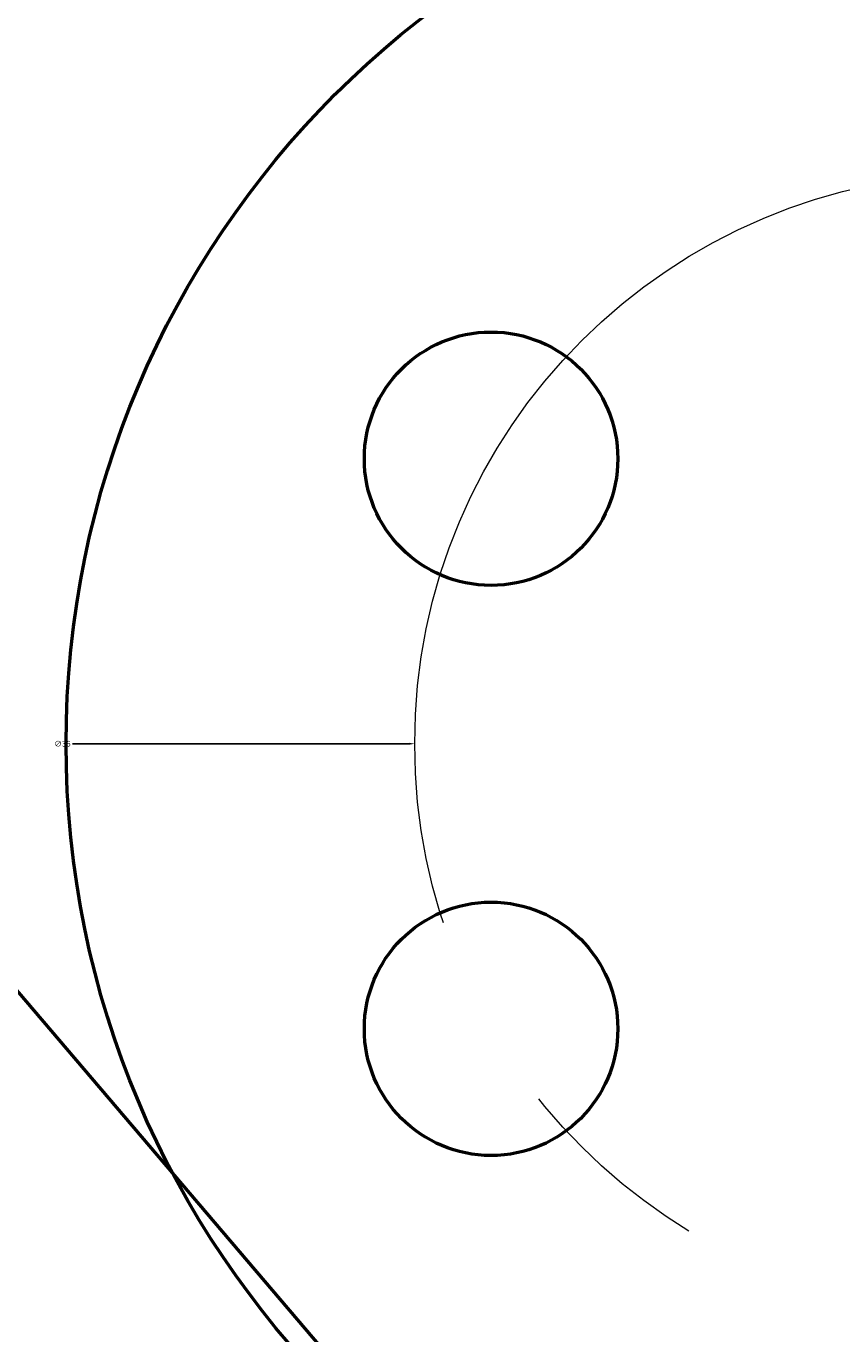
# Model space of a CAD drawing. Units: inches. Extents: x -11 to 126, y -62 to 82.
# Tile 3 of 10: x 29 to 55, y -40 to 1. Entities that reach past the tile are written whole.
import ezdxf

# ---------------------------------------------------------------- set-up
doc = ezdxf.new("R2010")
doc.units = ezdxf.units.IN
doc.header["$MEASUREMENT"] = 0
doc.linetypes.add('CENTER', pattern=[50.8, 31.75, -6.35, 6.35, -6.35])
for name, color, linetype, lineweight in [('M-CNTR', 4, 'CENTER', 18), ('M-DIMS', 2, 'Continuous', 18), ('M-OUTL', 7, 'Continuous', 50)]:
    doc.layers.add(name, color=color, linetype=linetype, lineweight=lineweight)
doc.styles.get("Standard").update_dxf_attribs({"font": 'arial.ttf'})
doc.dimstyles.get("Standard").update_dxf_attribs({"dimtxt": 0.18, "dimasz": 0.18, "dimexe": 0.18, "dimexo": 0.0625, "dimgap": 0.09, "dimtad": 0, "dimtih": 1, "dimtoh": 1, "dimdec": 4, "dimzin": 0, "dimdsep": 46, "dimtxsty": 'Standard', "dimcen": 0.09, "dimadec": 0, "dimazin": 0, "dimtfac": 1, "dimtdec": 4, "dimtofl": 0, "dimtmove": 0, "dimatfit": 3, "dimfxl": 1, "dimtolj": 1, "dimtzin": 0, "dimarcsym": 0})

# ---------------------------------------------------------------- blocks, each defined once
blk = doc.blocks.new('*U3')
blk.add_circle((0, 0), 4)
blk = doc.blocks.new('*U4')
at = {"layer": 'M-OUTL', "color": 0, "linetype": 'ByBlock', "lineweight": -2, "transparency": 16777216}
for p, rotation in [((43.643, -12.646), 59.99999999999999), ((43.643, -30.646), 120)]:
    blk.add_blockref('*U3', p, dxfattribs=dict(at, rotation=rotation))
blk = doc.blocks.new('*D5')
at = {"layer": 'Defpoints', "color": 0, "transparency": 16777216}
for p in [(119.232, 12.354), (-0.749, 11.479), (119.232, -57.296)]:
    blk.add_point(p, dxfattribs=at)
at = {"layer": 'M-DIMS', "color": 0, "lineweight": -2, "transparency": 16777216}
for p, q in [((119.232, 12.292), (119.232, -57.476)), ((-0.749, 11.416), (-0.749, -57.476)), ((-0.569, -57.296), (58.786, -57.296)), ((119.052, -57.296), (59.696, -57.296))]:
    blk.add_line(p, q, dxfattribs=at)
at = {"layer": 'M-DIMS', "color": 0, "transparency": 16777216}
for points in [[(-0.569, -57.266), (-0.569, -57.326), (-0.749, -57.296)], [(119.052, -57.266), (119.052, -57.326), (119.232, -57.296)]]:
    blk.add_solid(points, dxfattribs=at)
at = {"layer": 'M-DIMS', "color": 0, "transparency": 16777216, "insert": (59.241, -57.296), "char_height": 0.18, "attachment_point": 5}
blk.add_mtext('\\A1;119.98', dxfattribs=at)
blk = doc.blocks.new('*D6')
at = {"layer": 'Defpoints', "color": 0, "transparency": 16777216}
for p in [(-7.399, 75.354), (59.232, 75.354), (59.232, -50.646)]:
    blk.add_point(p, dxfattribs=at)
at = {"layer": 'M-DIMS', "color": 0, "lineweight": -2, "transparency": 16777216}
for p, q in [((59.169, 75.354), (-7.579, 75.354)), ((-7.399, 75.174), (-7.399, 12.536)), ((-7.399, -50.466), (-7.399, 12.172)), ((59.169, -50.646), (-7.579, -50.646))]:
    blk.add_line(p, q, dxfattribs=at)
at = {"layer": 'M-DIMS', "color": 0, "transparency": 16777216}
for points in [[(-7.429, 75.174), (-7.369, 75.174), (-7.399, 75.354)], [(-7.429, -50.466), (-7.369, -50.466), (-7.399, -50.646)]]:
    blk.add_solid(points, dxfattribs=at)
at = {"layer": 'M-DIMS', "color": 0, "transparency": 16777216, "insert": (-7.399, 12.354), "char_height": 0.18, "attachment_point": 5}
blk.add_mtext('\\A1;126', dxfattribs=at)
blk = doc.blocks.new('*D13')
at = {"layer": 'Defpoints', "color": 0, "transparency": 16777216}
for p in [(73.731, 3.469), (44.732, -46.761)]:
    blk.add_point(p, dxfattribs=at)
at = {"layer": 'M-DIMS', "color": 0, "lineweight": -2, "transparency": 16777216}
for p, q in [((59.142, -21.646), (59.322, -21.646)), ((59.232, -21.736), (59.232, -21.556)), ((36.032, -61.83), (44.642, -46.917)), ((35.852, -61.83), (36.032, -61.83))]:
    blk.add_line(p, q, dxfattribs=at)
at = {"layer": 'M-DIMS', "color": 0, "transparency": 16777216}
blk.add_solid([(44.616, -46.902), (44.668, -46.932), (44.732, -46.761)], dxfattribs=at)
at = {"layer": 'M-DIMS', "color": 0, "transparency": 16777216, "insert": (35.345, -61.83), "char_height": 0.18, "attachment_point": 5}
blk.add_mtext('\\A1;2X ∅58', dxfattribs=at)
blk = doc.blocks.new('*D15')
at = {"layer": 'Defpoints', "color": 0, "transparency": 16777216}
for p in [(41.232, -21.646), (77.232, -21.645)]:
    blk.add_point(p, dxfattribs=at)
at = {"layer": 'M-DIMS', "color": 0, "lineweight": -2, "transparency": 16777216}
for p, q in [((30.432, -21.646), (41.052, -21.646)), ((59.142, -21.646), (59.322, -21.646)), ((59.232, -21.736), (59.232, -21.556))]:
    blk.add_line(p, q, dxfattribs=at)
at = {"layer": 'M-DIMS', "color": 0, "transparency": 16777216}
blk.add_solid([(41.052, -21.616), (41.052, -21.676), (41.232, -21.646)], dxfattribs=at)
at = {"layer": 'M-DIMS', "color": 0, "transparency": 16777216, "insert": (30.115, -21.646), "char_height": 0.18, "attachment_point": 5}
blk.add_mtext('\\A1;∅36', dxfattribs=at)

msp = doc.modelspace()

# ---------------------------------------------------------------- linework, layer by layer
at = {"layer": 'M-CNTR'}
msp.add_circle((59.232, -21.646), 18, dxfattribs=at)
at = {"layer": 'M-OUTL'}
msp.add_line((3.002, 0.666), (41.77, -44.799), dxfattribs=at)
msp.add_circle((59.232, -21.646), 29, dxfattribs=at)

# ---------------------------------------------------------------- block references
msp.add_blockref('*U4', (0, 0), dxfattribs=at)

# ---------------------------------------------------------------- dimensions: what is measured, and where the dimension line sits
at = {"layer": 'M-DIMS'}
dim = msp.add_linear_dim(base=(-7.399, 75.354), p1=(59.232, -50.646), p2=(59.232, 75.354), angle=90, dimstyle='Standard', override={"dimdec": 0, "dimlfac": 1, "dimrnd": 0, "dimzin": 0, "dimdsep": 46, "dimlunit": 2}, dxfattribs=at)
dim.commit()
dim.dimension.update_dxf_attribs({"geometry": '*D6', "text_midpoint": (-7.399, 12.354)})
dim = msp.add_linear_dim(base=(119.232, -57.296), p1=(-0.749, 11.479), p2=(119.232, 12.354), dimstyle='Standard', override={"dimdec": 2, "dimlfac": 1, "dimrnd": 0, "dimzin": 0, "dimdsep": 46, "dimlunit": 2}, dxfattribs=at)
dim.commit()
dim.dimension.update_dxf_attribs({"geometry": '*D5', "text_midpoint": (59.241, -57.296)})
dim = msp.add_diameter_dim_2p(p1=(73.731, 3.469), p2=(44.732, -46.761), text='2X <>', dimstyle='Standard', override={"dimdec": 0, "dimlfac": 1, "dimrnd": 0, "dimzin": 0, "dimdsep": 46, "dimlunit": 2}, dxfattribs=at)
dim.commit()
dim.dimension.update_dxf_attribs({"geometry": '*D13', "text_midpoint": (35.345, -61.83), "dimtype": 163})
dim = msp.add_diameter_dim_2p(p1=(77.232, -21.645), p2=(41.232, -21.646), dimstyle='Standard', override={"dimdec": 0, "dimlfac": 1, "dimrnd": 0, "dimzin": 0, "dimdsep": 46, "dimlunit": 2}, dxfattribs=at)
dim.commit()
dim.dimension.update_dxf_attribs({"geometry": '*D15', "text_midpoint": (30.432, -21.646), "dimtype": 163})

doc.saveas('drawing.dxf')
